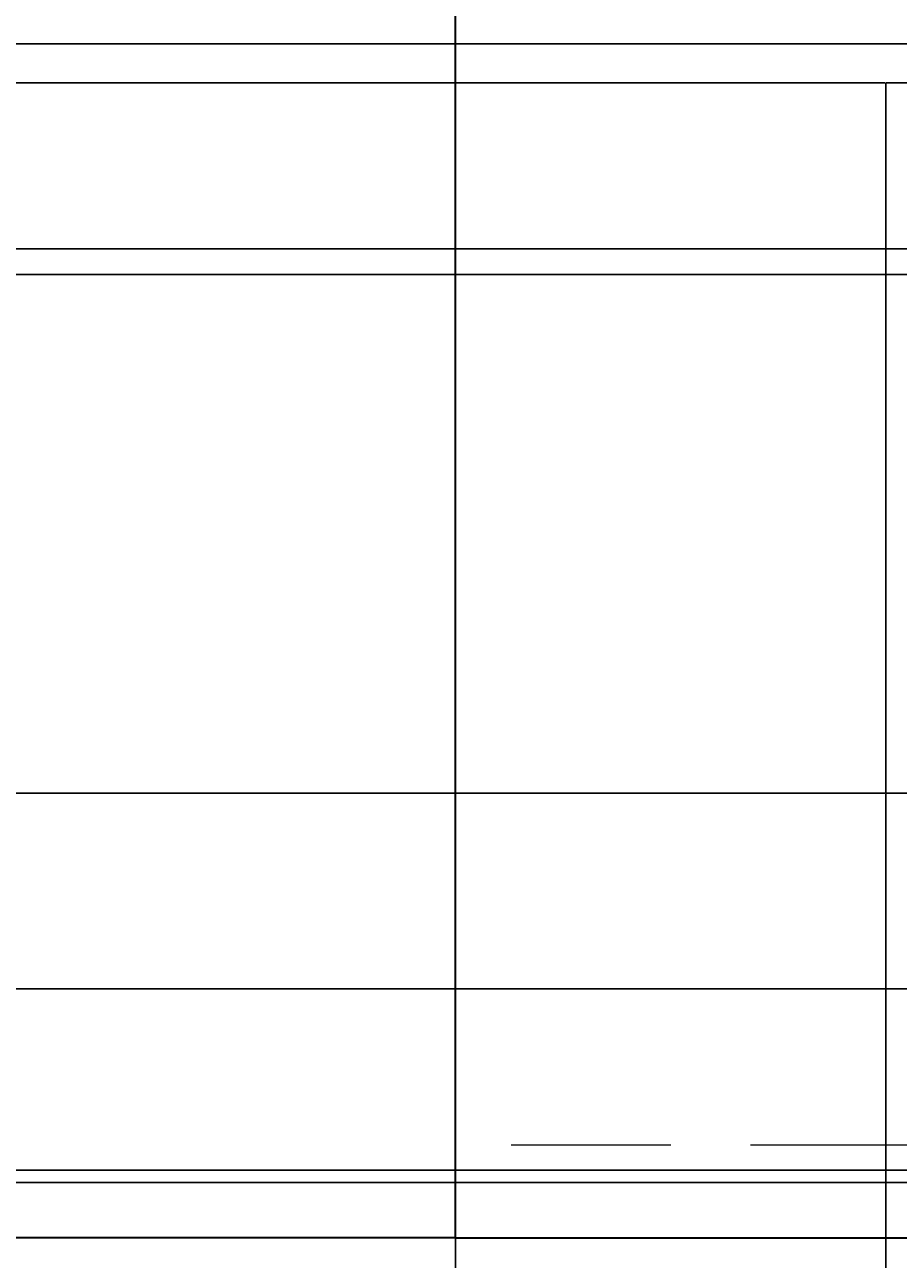
# Model space of a CAD drawing. Units: inches. Extents: x -145 to 510, y 5 to 386.
# Tile 5 of 25: x 20 to 89, y 78 to 177. Entities that reach past the tile are written whole.
import ezdxf

# ---------------------------------------------------------------- set-up
doc = ezdxf.new("R2010")
doc.units = ezdxf.units.IN
doc.header["$MEASUREMENT"] = 0
doc.linetypes.add('DASHED', pattern=[19.05, 12.7, -6.35])
for name, color, linetype, lineweight in [('A-ANNO-DIMS', 2, 'Continuous', 18), ('A-ELEV', 7, 'Continuous', 35), ('A-ELEV-HIDN', 8, 'DASHED', 18), ('A-GLAZ', 4, 'Continuous', 25)]:
    doc.layers.add(name, color=color, linetype=linetype, lineweight=lineweight)
doc.styles.get("Standard").update_dxf_attribs({"font": 'arial.ttf'})
doc.dimstyles.get("Standard").update_dxf_attribs({"dimtxt": 0.6875, "dimasz": 0.18, "dimexe": 0.18, "dimexo": 0.0625, "dimgap": 0.09, "dimtad": 0, "dimtih": 1, "dimtoh": 1, "dimdec": 4, "dimzin": 0, "dimdsep": 46, "dimlunit": 4, "dimtxsty": 'Standard', "dimcen": 0.09, "dimadec": 0, "dimazin": 0, "dimtfac": 1, "dimtdec": 4, "dimtofl": 0, "dimtmove": 0, "dimatfit": 3, "dimfxl": 1, "dimtolj": 1, "dimtzin": 0, "dimarcsym": 0})

# ---------------------------------------------------------------- blocks, each defined once
blk = doc.blocks.new('*D7')
at = {"layer": 'A-ANNO-DIMS', "color": 0, "lineweight": -2, "transparency": 16777216}
for p, q in [((88.246, 115.23), (88.246, 5.194)), ((54.001, 79.828), (54.001, 5.194)), ((54.181, 5.374), (69.604, 5.374)), ((88.066, 5.374), (72.643, 5.374))]:
    blk.add_line(p, q, dxfattribs=at)
at = {"layer": 'A-ANNO-DIMS', "color": 0, "transparency": 16777216}
for points in [[(54.181, 5.404), (54.181, 5.344), (54.001, 5.374)], [(88.066, 5.404), (88.066, 5.344), (88.246, 5.374)]]:
    blk.add_solid(points, dxfattribs=at)
at = {"layer": 'Defpoints', "color": 0, "transparency": 16777216}
for p in [(88.246, 115.292), (54.001, 79.891), (88.246, 5.374)]:
    blk.add_point(p, dxfattribs=at)
at = {"layer": 'A-ANNO-DIMS', "color": 0, "transparency": 16777216, "insert": (71.124, 5.374), "char_height": 0.6875, "attachment_point": 5}
blk.add_mtext('\\A1;34.245', dxfattribs=at)
blk = doc.blocks.new('*D8')
at = {"layer": 'A-ANNO-DIMS', "color": 0, "lineweight": -2, "transparency": 16777216}
for p, q in [((88.246, 115.23), (88.246, 5.194)), ((159.649, 115.23), (159.649, 5.194)), ((88.426, 5.374), (122.969, 5.374)), ((159.469, 5.374), (124.926, 5.374))]:
    blk.add_line(p, q, dxfattribs=at)
at = {"layer": 'A-ANNO-DIMS', "color": 0, "transparency": 16777216}
for points in [[(88.426, 5.404), (88.426, 5.344), (88.246, 5.374)], [(159.469, 5.404), (159.469, 5.344), (159.649, 5.374)]]:
    blk.add_solid(points, dxfattribs=at)
at = {"layer": 'Defpoints', "color": 0, "transparency": 16777216}
for p in [(88.246, 115.292), (159.649, 115.292), (159.649, 5.374)]:
    blk.add_point(p, dxfattribs=at)
at = {"layer": 'A-ANNO-DIMS', "color": 0, "transparency": 16777216, "insert": (123.948, 5.374), "char_height": 0.6875, "attachment_point": 5}
blk.add_mtext('\\A1;71.4', dxfattribs=at)
blk = doc.blocks.new('*D19')
at = {"layer": 'A-ANNO-DIMS', "color": 0, "lineweight": -2, "transparency": 16777216}
for p, q in [((478.764, 355.891), (-144.054, 355.891)), ((-143.874, 355.711), (-143.874, 218.332)), ((-143.874, 80.071), (-143.874, 217.45)), ((-114.036, 79.891), (-144.054, 79.891))]:
    blk.add_line(p, q, dxfattribs=at)
at = {"layer": 'A-ANNO-DIMS', "color": 0, "transparency": 16777216}
for points in [[(-143.904, 355.711), (-143.844, 355.711), (-143.874, 355.891)], [(-143.904, 80.071), (-143.844, 80.071), (-143.874, 79.891)]]:
    blk.add_solid(points, dxfattribs=at)
at = {"layer": 'Defpoints', "color": 0, "transparency": 16777216}
for p in [(-143.874, 355.891), (478.826, 355.891), (-113.974, 79.891)]:
    blk.add_point(p, dxfattribs=at)
at = {"layer": 'A-ANNO-DIMS', "color": 0, "transparency": 16777216, "insert": (-143.874, 217.891), "char_height": 0.6875, "attachment_point": 5}
blk.add_mtext('\\A1;276', dxfattribs=at)
blk = doc.blocks.new('*D20')
at = {"layer": 'A-ANNO-DIMS', "color": 0, "lineweight": -2, "transparency": 16777216}
for p, q in [((53.939, 199.891), (-144.054, 199.891)), ((-143.874, 199.711), (-143.874, 140.332)), ((-143.874, 80.071), (-143.874, 139.45)), ((53.939, 79.891), (-144.054, 79.891))]:
    blk.add_line(p, q, dxfattribs=at)
at = {"layer": 'A-ANNO-DIMS', "color": 0, "transparency": 16777216}
for points in [[(-143.904, 199.711), (-143.844, 199.711), (-143.874, 199.891)], [(-143.904, 80.071), (-143.844, 80.071), (-143.874, 79.891)]]:
    blk.add_solid(points, dxfattribs=at)
at = {"layer": 'Defpoints', "color": 0, "transparency": 16777216}
for p in [(-143.874, 199.891), (54.001, 199.891), (54.001, 79.891)]:
    blk.add_point(p, dxfattribs=at)
at = {"layer": 'A-ANNO-DIMS', "color": 0, "transparency": 16777216, "insert": (-143.874, 139.891), "char_height": 0.6875, "attachment_point": 5}
blk.add_mtext('\\A1;120', dxfattribs=at)
blk = doc.blocks.new('*D23')
at = {"layer": 'A-ANNO-DIMS', "color": 0, "lineweight": -2, "transparency": 16777216}
for p, q in [((88.184, 115.292), (-144.054, 115.292)), ((-143.874, 115.112), (-143.874, 98.033)), ((-143.874, 80.071), (-143.874, 97.15)), ((53.939, 79.891), (-144.054, 79.891))]:
    blk.add_line(p, q, dxfattribs=at)
at = {"layer": 'A-ANNO-DIMS', "color": 0, "transparency": 16777216}
for points in [[(-143.904, 115.112), (-143.844, 115.112), (-143.874, 115.292)], [(-143.904, 80.071), (-143.844, 80.071), (-143.874, 79.891)]]:
    blk.add_solid(points, dxfattribs=at)
at = {"layer": 'Defpoints', "color": 0, "transparency": 16777216}
for p in [(-143.874, 115.292), (88.246, 115.292), (54.001, 79.891)]:
    blk.add_point(p, dxfattribs=at)
at = {"layer": 'A-ANNO-DIMS', "color": 0, "transparency": 16777216, "insert": (-143.874, 97.591), "char_height": 0.6875, "attachment_point": 5}
blk.add_mtext('\\A1;35.4', dxfattribs=at)
blk = doc.blocks.new('*D24')
at = {"layer": 'A-ANNO-DIMS', "color": 0, "lineweight": -2, "transparency": 16777216}
for p, q in [((88.184, 171.872), (-144.054, 171.872)), ((-143.874, 171.692), (-143.874, 144.023)), ((-143.874, 115.472), (-143.874, 143.141)), ((88.184, 115.292), (-144.054, 115.292))]:
    blk.add_line(p, q, dxfattribs=at)
at = {"layer": 'A-ANNO-DIMS', "color": 0, "transparency": 16777216}
for points in [[(-143.904, 171.692), (-143.844, 171.692), (-143.874, 171.872)], [(-143.904, 115.472), (-143.844, 115.472), (-143.874, 115.292)]]:
    blk.add_solid(points, dxfattribs=at)
at = {"layer": 'Defpoints', "color": 0, "transparency": 16777216}
for p in [(-143.874, 171.872), (88.246, 171.872), (88.246, 115.292)]:
    blk.add_point(p, dxfattribs=at)
at = {"layer": 'A-ANNO-DIMS', "color": 0, "transparency": 16777216, "insert": (-143.874, 143.582), "char_height": 0.6875, "attachment_point": 5}
blk.add_mtext('\\A1;56.58', dxfattribs=at)
blk = doc.blocks.new('*D29')
at = {"layer": 'A-ANNO-DIMS', "color": 0, "lineweight": -2, "transparency": 16777216}
for p, q in [((221.467, 174.992), (-144.054, 174.992)), ((-143.874, 174.812), (-143.874, 130.569)), ((-143.874, 85.444), (-143.874, 129.687)), ((221.467, 85.264), (-144.054, 85.264))]:
    blk.add_line(p, q, dxfattribs=at)
at = {"layer": 'A-ANNO-DIMS', "color": 0, "transparency": 16777216}
for points in [[(-143.904, 174.812), (-143.844, 174.812), (-143.874, 174.992)], [(-143.904, 85.444), (-143.844, 85.444), (-143.874, 85.264)]]:
    blk.add_solid(points, dxfattribs=at)
at = {"layer": 'Defpoints', "color": 0, "transparency": 16777216}
for p in [(-143.874, 174.992), (221.529, 174.992), (221.529, 85.264)]:
    blk.add_point(p, dxfattribs=at)
at = {"layer": 'A-ANNO-DIMS', "color": 0, "transparency": 16777216, "insert": (-143.874, 130.128), "char_height": 0.6875, "attachment_point": 5}
blk.add_mtext('\\A1;89.73', dxfattribs=at)
blk = doc.blocks.new('*D41')
at = {"layer": 'A-ANNO-DIMS', "color": 0, "lineweight": -2, "transparency": 16777216}
for p, q in [((15.744, 109.056), (15.744, 5.194)), ((54.001, 79.828), (54.001, 5.194)), ((15.924, 5.374), (33.623, 5.374)), ((53.821, 5.374), (36.122, 5.374))]:
    blk.add_line(p, q, dxfattribs=at)
at = {"layer": 'A-ANNO-DIMS', "color": 0, "transparency": 16777216}
for points in [[(15.924, 5.404), (15.924, 5.344), (15.744, 5.374)], [(53.821, 5.404), (53.821, 5.344), (54.001, 5.374)]]:
    blk.add_solid(points, dxfattribs=at)
at = {"layer": 'Defpoints', "color": 0, "transparency": 16777216}
for p in [(15.744, 109.118), (54.001, 79.891), (54.001, 5.374)]:
    blk.add_point(p, dxfattribs=at)
at = {"layer": 'A-ANNO-DIMS', "color": 0, "transparency": 16777216, "insert": (34.873, 5.374), "char_height": 0.6875, "attachment_point": 5}
blk.add_mtext('\\A1;38.26', dxfattribs=at)
blk = doc.blocks.new('*D54')
at = {"layer": 'A-ANNO-DIMS', "color": 0, "lineweight": -2, "transparency": 16777216}
for p, q in [((315.492, 156.609), (-144.054, 156.609)), ((-143.874, 156.429), (-143.874, 121.378)), ((-143.874, 85.444), (-143.874, 120.495)), ((315.492, 85.264), (-144.054, 85.264))]:
    blk.add_line(p, q, dxfattribs=at)
at = {"layer": 'A-ANNO-DIMS', "color": 0, "transparency": 16777216}
for points in [[(-143.904, 156.429), (-143.844, 156.429), (-143.874, 156.609)], [(-143.904, 85.444), (-143.844, 85.444), (-143.874, 85.264)]]:
    blk.add_solid(points, dxfattribs=at)
at = {"layer": 'Defpoints', "color": 0, "transparency": 16777216}
for p in [(-143.874, 156.609), (315.554, 156.609), (315.554, 85.264)]:
    blk.add_point(p, dxfattribs=at)
at = {"layer": 'A-ANNO-DIMS', "color": 0, "transparency": 16777216, "insert": (-143.874, 120.937), "char_height": 0.6875, "attachment_point": 5}
blk.add_mtext('\\A1;71.35', dxfattribs=at)
blk = doc.blocks.new('*D55')
at = {"layer": 'A-ANNO-DIMS', "color": 0, "lineweight": -2, "transparency": 16777216}
for p, q in [((314.432, 174.992), (-144.054, 174.992)), ((-143.874, 174.812), (-143.874, 167.266)), ((-143.874, 158.837), (-143.874, 166.383)), ((314.432, 158.657), (-144.054, 158.657))]:
    blk.add_line(p, q, dxfattribs=at)
at = {"layer": 'A-ANNO-DIMS', "color": 0, "transparency": 16777216}
for points in [[(-143.904, 174.812), (-143.844, 174.812), (-143.874, 174.992)], [(-143.904, 158.837), (-143.844, 158.837), (-143.874, 158.657)]]:
    blk.add_solid(points, dxfattribs=at)
at = {"layer": 'Defpoints', "color": 0, "transparency": 16777216}
for p in [(-143.874, 174.992), (314.494, 174.992), (314.494, 158.657)]:
    blk.add_point(p, dxfattribs=at)
at = {"layer": 'A-ANNO-DIMS', "color": 0, "transparency": 16777216, "insert": (-143.874, 166.825), "char_height": 0.6875, "attachment_point": 5}
blk.add_mtext('\\A1;16.335', dxfattribs=at)
blk = doc.blocks.new('*D57')
at = {"layer": 'A-ANNO-DIMS', "color": 0, "lineweight": -2, "transparency": 16777216}
for p, q in [((263.856, 99.712), (-144.054, 99.712)), ((-143.874, 99.532), (-143.874, 92.436)), ((-143.874, 84.459), (-143.874, 91.554)), ((271.428, 84.279), (-144.054, 84.279))]:
    blk.add_line(p, q, dxfattribs=at)
at = {"layer": 'A-ANNO-DIMS', "color": 0, "transparency": 16777216}
for points in [[(-143.904, 99.532), (-143.844, 99.532), (-143.874, 99.712)], [(-143.904, 84.459), (-143.844, 84.459), (-143.874, 84.279)]]:
    blk.add_solid(points, dxfattribs=at)
at = {"layer": 'Defpoints', "color": 0, "transparency": 16777216}
for p in [(-143.874, 99.712), (263.918, 99.712), (271.491, 84.279)]:
    blk.add_point(p, dxfattribs=at)
at = {"layer": 'A-ANNO-DIMS', "color": 0, "transparency": 16777216, "insert": (-143.874, 91.995), "char_height": 0.6875, "attachment_point": 5}
blk.add_mtext('\\A1;15.433', dxfattribs=at)

msp = doc.modelspace()

# ---------------------------------------------------------------- linework, layer by layer
at = {"layer": 'A-ELEV'}
for q in [(54.0014, 199.8905), (-113.9737, 79.8905), (392.4492, 79.8905)]:
    msp.add_line((54.0014, 79.8905), q, dxfattribs=at)
at = {"layer": 'A-ELEV-HIDN'}
msp.add_line((223.5292, 87.2638), (54.0014, 87.2638), dxfattribs=at)
at = {"layer": 'A-GLAZ'}
msp.add_lwpolyline([(88.2462, 171.8717), (159.6492, 171.8717), (159.6492, 115.2922), (88.2462, 115.2922)], close=True, dxfattribs=at)

# ---------------------------------------------------------------- dimensions: what is measured, and where the dimension line sits
at = {"layer": 'A-ANNO-DIMS'}
for base, p1, p2, override, picture, middle in [((-143.8737, 355.8905), (-113.9737, 79.8905), (478.8263, 355.8905), {"dimdec": 0, "dimlfac": 1, "dimrnd": 0, "dimzin": 0, "dimdsep": 46, "dimlunit": 2}, '*D19', (-143.8737, 217.8905)), ((-143.8737, 199.8905), (54.0014, 79.8905), (54.0014, 199.8905), {"dimdec": 0, "dimlfac": 1, "dimrnd": 0, "dimzin": 0, "dimdsep": 46, "dimlunit": 2}, '*D20', (-143.8737, 139.8905)), ((-143.8737, 174.9923), (314.494, 158.657), (314.494, 174.9923), {"dimdec": 3, "dimlfac": 1, "dimrnd": 0, "dimzin": 0, "dimdsep": 46, "dimlunit": 2}, '*D55', (-143.8737, 166.8247)), ((-143.8737, 174.9923), (221.5292, 85.2638), (221.5292, 174.9923), {"dimdec": 2, "dimlfac": 1, "dimrnd": 0, "dimzin": 0, "dimdsep": 46, "dimlunit": 2}, '*D29', (-143.8737, 130.1281)), ((-143.8737, 171.8717), (88.2462, 115.2922), (88.2462, 171.8717), {"dimdec": 2, "dimlfac": 1, "dimrnd": 0, "dimzin": 0, "dimdsep": 46, "dimlunit": 2}, '*D24', (-143.8737, 143.5819)), ((-143.8737, 156.6093), (315.5545, 85.2638), (315.5545, 156.6093), {"dimdec": 2, "dimlfac": 1, "dimrnd": 0, "dimzin": 0, "dimdsep": 46, "dimlunit": 2}, '*D54', (-143.8737, 120.9365)), ((-143.8737, 115.2922), (54.0014, 79.8905), (88.2462, 115.2922), {"dimdec": 1, "dimlfac": 1, "dimrnd": 0, "dimzin": 0, "dimdsep": 46, "dimlunit": 2}, '*D23', (-143.8737, 97.5914)), ((-143.8737, 99.7118), (271.4905, 84.2785), (263.9183, 99.7118), {"dimdec": 3, "dimlfac": 1, "dimrnd": 0, "dimzin": 0, "dimdsep": 46, "dimlunit": 2}, '*D57', (-143.8737, 91.9952))]:
    dim = msp.add_linear_dim(base=base, p1=p1, p2=p2, angle=90, dimstyle='Standard', override=override, dxfattribs=at)
    dim.commit()
    dim.dimension.update_dxf_attribs({"geometry": picture, "text_midpoint": middle})
for base, p1, p2, override, picture, middle in [((88.2462, 5.3738), (54.0014, 79.8905), (88.2462, 115.2922), {"dimdec": 3, "dimlfac": 1, "dimrnd": 0, "dimzin": 0, "dimdsep": 46, "dimlunit": 2}, '*D7', (71.1238, 5.3738)), ((159.6492, 5.3738), (88.2462, 115.2922), (159.6492, 115.2922), {"dimdec": 1, "dimlfac": 1, "dimrnd": 0, "dimzin": 0, "dimdsep": 46, "dimlunit": 2}, '*D8', (123.9477, 5.3738)), ((54.0014, 5.3738), (15.7444, 109.1183), (54.0014, 79.8905), {"dimdec": 2, "dimlfac": 1, "dimrnd": 0, "dimzin": 0, "dimdsep": 46, "dimlunit": 2}, '*D41', (34.8729, 5.3738))]:
    dim = msp.add_linear_dim(base=base, p1=p1, p2=p2, dimstyle='Standard', override=override, dxfattribs=at)
    dim.commit()
    dim.dimension.update_dxf_attribs({"geometry": picture, "text_midpoint": middle})

doc.saveas('drawing.dxf')
